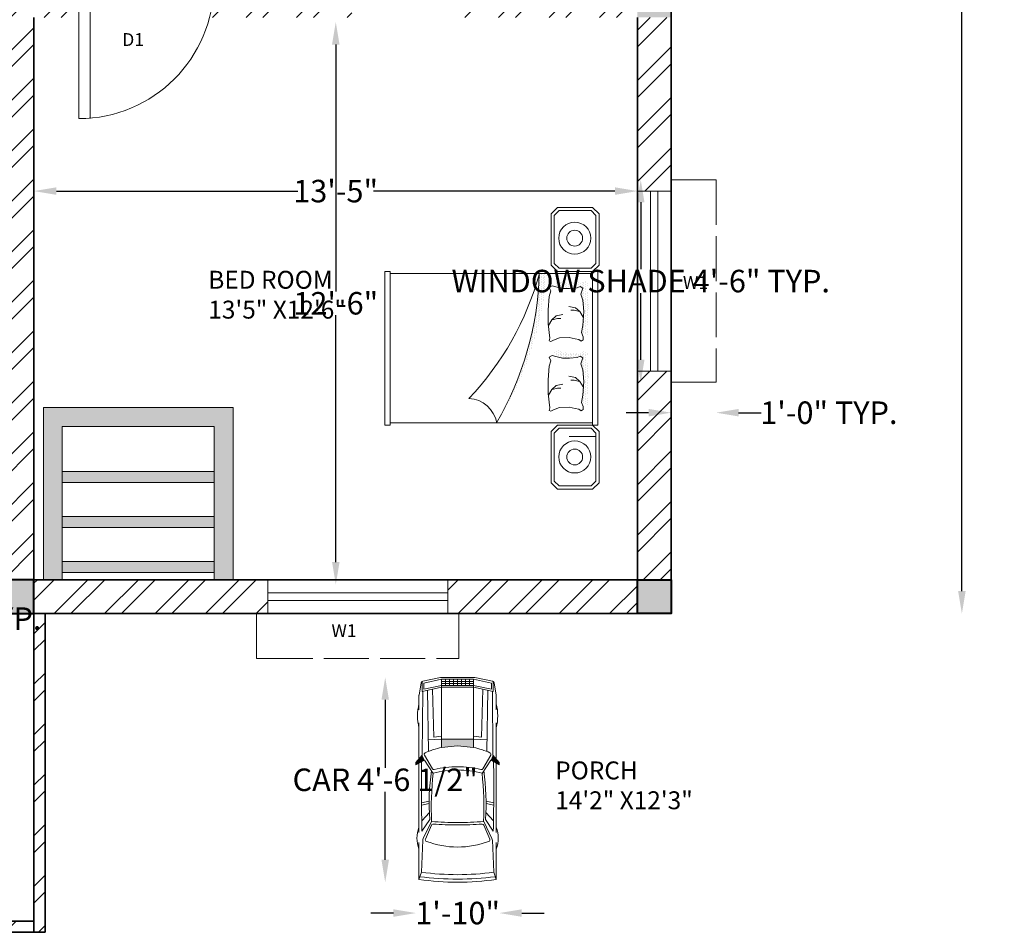
# Model space of a CAD drawing. Units: inches. Extents: x 3614 to 4242, y 2406 to 3033.
# Tile 9 of 10: x 3980 to 4242, y 2489 to 2733. Entities that reach past the tile are written whole.
import ezdxf

# ---------------------------------------------------------------- set-up
doc = ezdxf.new("R2010")
doc.units = ezdxf.units.IN
doc.linetypes.add('ACAD_ISO02W100', pattern=[15, 12, -3])
for name, color, linetype, lineweight in [('A-ANNO-DIMS', 2, 'Continuous', 18), ('A-ANNO-TEXT', 7, 'Continuous', 18), ('A-AREA-IDEN', 7, 'Continuous', 25), ('A-COLS', 7, 'Continuous', 40), ('A-COLS-PATT', 252, 'Continuous', 18), ('A-DOOR', 3, 'Continuous', 18), ('A-EQPM', 8, 'Continuous', 18), ('A-FURN', 8, 'Continuous', 18), ('A-FURN-PATT', 252, 'Continuous', 13), ('A-GLAZ', 4, 'Continuous', 18), ('A-GLAZ-OVHD', 8, 'ACAD_ISO02W100', 13), ('A-WALL', 7, 'Continuous', 35), ('A-WALL-PATT', 252, 'Continuous', 13)]:
    doc.layers.add(name, color=color, linetype=linetype, lineweight=lineweight)
doc.styles.add('ATTR', font='romans.shx', dxfattribs={"width": 0.8, "height": 1.114828})
doc.styles.get("Standard").update_dxf_attribs({"font": 'arial.ttf'})
doc.dimstyles.get("Standard").update_dxf_attribs({"dimtxt": 6, "dimasz": 6, "dimexe": 0.18, "dimexo": 0.0625, "dimgap": 0.09, "dimtad": 0, "dimtih": 1, "dimtoh": 1, "dimdec": 4, "dimzin": 0, "dimdsep": 46, "dimlunit": 4, "dimtxsty": 'Standard', "dimcen": 0.09, "dimse1": 1, "dimse2": 1, "dimadec": 0, "dimazin": 0, "dimtfac": 1, "dimtdec": 4, "dimtofl": 0, "dimtmove": 0, "dimatfit": 3, "dimfxl": 1, "dimtolj": 1, "dimtzin": 0, "dimarcsym": 0})
pattern_1 = [(270, (-3578.6833, 5895.14276), (0.451673685, -0.225836843), [0, -0.451673685])]

# ---------------------------------------------------------------- blocks, each defined once
blk = doc.blocks.new('*D19')
at = {"layer": 'A-ANNO-DIMS', "color": 0, "lineweight": -2, "transparency": 16777216}
for p, q in [((4063.88, 2726.09), (4063.88, 2660.24)), ((4063.88, 2588.09), (4063.88, 2653.94))]:
    blk.add_line(p, q, dxfattribs=at)
at = {"layer": 'A-ANNO-DIMS', "color": 0, "transparency": 16777216}
for points in [[(4062.88, 2726.09), (4064.88, 2726.09), (4063.88, 2732.09)], [(4062.88, 2588.09), (4064.88, 2588.09), (4063.88, 2582.09)]]:
    blk.add_solid(points, dxfattribs=at)
at = {"layer": 'Defpoints', "color": 0, "transparency": 16777216}
for p in [(4096.83, 2732.09), (4063.88, 2582.09), (4096.83, 2582.09)]:
    blk.add_point(p, dxfattribs=at)
at = {"layer": 'A-ANNO-DIMS', "color": 0, "transparency": 16777216, "insert": (4063.88, 2657.09), "char_height": 6, "attachment_point": 5}
blk.add_mtext('\\A1;12\'-6"', dxfattribs=at)
blk = doc.blocks.new('*D20')
at = {"layer": 'A-ANNO-DIMS', "color": 0, "lineweight": -2, "transparency": 16777216}
for p, q in [((3989.34, 2687.01), (4053.72, 2687.01)), ((4138.34, 2687.01), (4073.95, 2687.01))]:
    blk.add_line(p, q, dxfattribs=at)
at = {"layer": 'A-ANNO-DIMS', "color": 0, "transparency": 16777216}
for points in [[(3989.34, 2688.01), (3989.34, 2686.01), (3983.34, 2687.01)], [(4138.34, 2688.01), (4138.34, 2686.01), (4144.34, 2687.01)]]:
    blk.add_solid(points, dxfattribs=at)
at = {"layer": 'Defpoints', "color": 0, "transparency": 16777216}
for p in [(3983.34, 2692), (4144.34, 2692), (4144.34, 2687.01)]:
    blk.add_point(p, dxfattribs=at)
at = {"layer": 'A-ANNO-DIMS', "color": 0, "transparency": 16777216, "insert": (4063.84, 2687.01), "char_height": 6, "attachment_point": 5}
blk.add_mtext('\\A1;13\'-5"', dxfattribs=at)
blk = doc.blocks.new('A$C682073C8')
for p, q in [((-1.51, 0.58), (-1.388, 0.684)), ((-1.428, 0.543), (-1.348, 0.684)), ((-1.388, 0.684), (-1.348, 0.684)), ((-2.78, 0.282), (-2.724, 0.571)), ((-2.69, 0.555), (-2.752, 0.263)), ((-2.554, 0.581), (-2.72, 0.581)), ((-2.694, 0.6), (-2.493, 0.633)), ((-2.59, 0.555), (-2.69, 0.555)), ((-2.59, 0.555), (-2.652, 0.263)), ((-2.554, 0.581), (-2.622, 0.263)), ((-1.57, 0.478), (-2.572, 0.496)), ((-2.557, 0.57), (-1.51, 0.58)), ((-2.251, 0.635), (-2.478, 0.635)), ((-1.445, 0.635), (-2.04, 0.635)), ((-1.286, 0.414), (-1.508, 0.544)), ((-1.209, 0.401), (-1.428, 0.543)), ((-0.237, 0.635), (-1.376, 0.635)), ((-0.755, 0.467), (-0.727, 0.593)), ((-0.714, 0.467), (-0.686, 0.593)), ((-0.432, 0.589), (-0.565, 0.464)), ((-0.451, 0.457), (-0.263, 0.585)), ((-0.142, 0.564), (-0.42, 0.428)), ((-0.361, 0.431), (-0.128, 0.528)), ((0.411, 0.593), (-0.11, 0.572)), ((0.532, 0.635), (-0.072, 0.635)), ((0.532, 0.635), (0.411, 0.593)), ((-1.805, 0.393), (-2.59, 0.413)), ((-1.818, 0.263), (-1.805, 0.393)), ((-1.771, 0.263), (-1.758, 0.481)), ((-2.781, 0), (-2.781, 0.273)), ((-2.752, 0.263), (-2.752, 0)), ((-1.633, 0.263), (-2.752, 0.263)), ((-2.652, 0.197), (-2.752, 0.197)), ((-2.718, 0.263), (-2.718, 0)), ((-2.685, 0.263), (-2.685, 0)), ((-2.652, 0.263), (-2.652, 0)), ((-2.622, 0.263), (-2.622, 0)), ((-1.771, 0.263), (-1.771, 0)), ((-1.633, 0.263), (-1.659, 0)), ((-2.781, 0), (-2.781, -0.273)), ((-2.652, 0.132), (-2.752, 0.132)), ((-2.652, 0.066), (-2.752, 0.066)), ((-2.652, 0), (-2.752, 0)), ((-2.752, -0.263), (-2.752, 0)), ((-2.718, -0.263), (-2.718, 0)), ((-2.685, -0.263), (-2.685, 0)), ((-2.652, -0.263), (-2.652, 0)), ((-2.622, -0.263), (-2.622, 0)), ((-1.771, -0.263), (-1.771, 0)), ((-1.659, 0), (-1.633, -0.263)), ((-2.652, -0.066), (-2.752, -0.066)), ((-2.652, -0.132), (-2.752, -0.132)), ((-2.78, -0.282), (-2.724, -0.571)), ((-2.652, -0.197), (-2.752, -0.197)), ((-1.633, -0.263), (-2.752, -0.263)), ((-2.69, -0.555), (-2.752, -0.263)), ((-2.59, -0.555), (-2.652, -0.263)), ((-2.554, -0.581), (-2.622, -0.263)), ((-1.818, -0.263), (-1.805, -0.393)), ((-1.771, -0.263), (-1.758, -0.481)), ((-1.805, -0.393), (-2.59, -0.413)), ((-1.57, -0.478), (-2.572, -0.496)), ((-1.286, -0.414), (-1.508, -0.544)), ((-1.209, -0.401), (-1.428, -0.543)), ((-0.755, -0.467), (-0.727, -0.593)), ((-0.714, -0.467), (-0.686, -0.593)), ((-0.432, -0.589), (-0.565, -0.464)), ((-0.451, -0.457), (-0.263, -0.585)), ((-0.142, -0.564), (-0.42, -0.428)), ((-0.361, -0.431), (-0.128, -0.528)), ((-2.554, -0.581), (-2.72, -0.581)), ((-2.694, -0.6), (-2.493, -0.633)), ((-2.59, -0.555), (-2.69, -0.555)), ((-2.557, -0.57), (-1.51, -0.58)), ((-2.251, -0.635), (-2.478, -0.635)), ((-1.445, -0.635), (-2.04, -0.635)), ((-1.51, -0.58), (-1.388, -0.684)), ((-1.428, -0.543), (-1.348, -0.684)), ((-0.237, -0.635), (-1.376, -0.635)), ((0.411, -0.593), (-0.11, -0.572)), ((0.532, -0.635), (-0.072, -0.635)), ((0.532, -0.635), (0.411, -0.593)), ((-1.388, -0.684), (-1.348, -0.684))]:
    blk.add_line(p, q)
for centre, radius, start, end in [((-2.154, -0.189), 0.847, 76.4679, 103.5321), ((-0.146, 0.162), 0.505, 69.2613, 110.7387), ((-2.688, 0.564), 0.0366, 99.5555, 168.9219), ((-2.478, 0.542), 0.0932, 90, 99.5555), ((-0.341, 0), 1.319, 156.2323, 168.4871), ((-1.522, 0.52), 0.0277, 59.6014, 156.2323), ((-0.97, -26.413), 27.007, 88.4985, 90.9138), ((-0.106, 0.49), 0.0817, 92.3222, 116.0777), ((-0.118, 0.504), 0.0264, 20.6689, 112.6283), ((-1.453, 0), 1.453, 360, 20.6689), ((-3.642, 0), 4.096, 360, 8.3245), ((-4.512, 0), 5.038, 360, 7.0662), ((-3.75, 0), 4.328, 360, 8.4328), ((0.324, 0), 1.642, 166.5017, 180), ((-1.3, 0.39), 0.0277, 346.5017, 59.6014), ((0.222, 0), 1.487, 164.3473, 180), ((-0.728, -3.189), 3.656, 85.6618, 98.2609), ((-0.642, -4.704), 5.136, 87.5218, 96.3432), ((-5.551, 0), 5.149, 360, 4.7655), ((-0.35, 0.407), 0.0264, 112.6283, 183.982), ((-6.195, 0), 5.833, 360, 3.982), ((-2.736, 0.273), 0.045, 168.9219, 180), ((0.324, 0), 1.642, 180, 193.4983), ((0.222, 0), 1.487, 180, 195.6527), ((-5.551, 0), 5.149, 355.2345, 360), ((-6.195, 0), 5.833, 356.018, 360), ((-1.453, 0), 1.453, 339.3311, 360), ((-3.642, 0), 4.096, 351.6755, 360), ((-4.512, 0), 5.038, 352.9338, 360), ((-3.75, 0), 4.328, 351.5672, 360), ((-2.736, -0.273), 0.045, 180, 191.0781), ((-0.341, 0), 1.319, 191.5129, 203.7677), ((-1.3, -0.39), 0.0277, 300.3986, 13.4983), ((-0.728, 3.189), 3.656, 261.7391, 274.3382), ((-0.642, 4.704), 5.136, 263.6568, 272.4781), ((-0.35, -0.407), 0.0264, 176.018, 247.3717), ((-2.688, -0.564), 0.0366, 191.0781, 260.4445), ((-2.478, -0.542), 0.0932, 260.4445, 270), ((-2.154, 0.189), 0.847, 256.4679, 283.5321), ((-1.522, -0.52), 0.0277, 203.7677, 300.3986), ((-0.97, 26.413), 27.007, 269.0862, 271.5015), ((-0.146, -0.162), 0.505, 249.2613, 290.7387), ((-0.106, -0.49), 0.0817, 243.9223, 267.6778), ((-0.118, -0.504), 0.0264, 247.3717, 339.3311)]:
    blk.add_arc(centre, radius, start, end)
for points in [[(-1.428, 0.543), (-1.51, 0.58), (-1.348, 0.684), (-1.388, 0.684)], [(-1.633, 0.263), (-1.659, 0), (-1.771, 0.263), (-1.771, -0.263)], [(-1.659, 0), (-1.633, -0.263), (-1.771, -0.263)], [(-1.428, -0.543), (-1.51, -0.58), (-1.348, -0.684), (-1.388, -0.684)]]:
    blk.add_solid(points)
at = {"style": 'ATTR', "width": 0.8, "flags": 9}
blk.add_attdef('ESTCODE', (-2.781, 0), '', height=0.00071, rotation=180, dxfattribs=at)
blk = doc.blocks.new('*D25')
at = {"layer": 'A-ANNO-DIMS', "color": 0, "lineweight": -2, "transparency": 16777216}
for p, q in [((4230.92, 2948.34), (4230.92, 2767.5)), ((4230.92, 2580.34), (4230.92, 2761.19))]:
    blk.add_line(p, q, dxfattribs=at)
at = {"layer": 'A-ANNO-DIMS', "color": 0, "transparency": 16777216}
for points in [[(4229.92, 2948.34), (4231.92, 2948.34), (4230.92, 2954.34)], [(4229.92, 2580.34), (4231.92, 2580.34), (4230.92, 2574.34)]]:
    blk.add_solid(points, dxfattribs=at)
at = {"layer": 'Defpoints', "color": 0, "transparency": 16777216}
for p in [(4153.34, 2954.34), (4153.34, 2574.34), (4230.92, 2574.34)]:
    blk.add_point(p, dxfattribs=at)
at = {"layer": 'A-ANNO-DIMS', "color": 0, "transparency": 16777216, "insert": (4230.92, 2764.34), "char_height": 6, "attachment_point": 5}
blk.add_mtext('\\A1;31\'-8"', dxfattribs=at)
blk = doc.blocks.new('WINDOW-W1-48IN')
for p, q in [((48, 9), (0, 9)), ((0, 9), (0, 0)), ((48, 0), (48, 9)), ((0, 5.5), (48, 5.5)), ((0, 3.5), (48, 3.5)), ((0, 0), (48, 0))]:
    blk.add_line(p, q)
blk = doc.blocks.new('SHADE-W1')
for p, q in [((0, 0), (0, 12)), ((0, 12), (51, 12)), ((51, 12), (54, 12)), ((54, 12), (54, 0)), ((3, 0), (0, 0))]:
    blk.add_line(p, q)
blk = doc.blocks.new('COLUMN-9X9')
blk.add_lwpolyline([(9, 9), (0, 9), (0, 0), (9, 0)], close=True)
blk = doc.blocks.new('DOOR-SWING-36IN')
for p, q in [((0, 36), (0, 0)), ((0, 0), (0, 36)), ((3, 0), (3, 36))]:
    blk.add_line(p, q)
blk.add_arc((0, 36), 36, 270, 0)
blk = doc.blocks.new('BED-DOUBLE-WITH-NIGHTSTANDS')
h = blk.add_hatch()
h.set_pattern_fill('DOTS', color=256, scale=0.284519, angle=-90, style=0)
h.set_pattern_definition(pattern_1)
h.paths.add_polyline_path([(43.21, 57.47), (41.26, 57.47, -0.124273), (29.87, 17.64, 0.122563)])
h = blk.add_hatch()
h.set_pattern_fill('DOTS', color=256, scale=0.284519, angle=-90, style=0)
h.set_pattern_definition(pattern_1)
h.paths.add_polyline_path([(53.82, 40.86), (54.34, 41.21), (54.34, 42), (53.9, 43.14), (54.25, 45.06), (54.52, 48.74), (54.25, 51.8), (53.73, 53.38), (54.25, 55.04), (53.55, 55.48), (52.77, 55.13), (50.75, 54.95), (48.83, 54.95), (47.08, 55.39), (46.12, 55.65), (45.33, 55.22), (45.77, 54.25), (45.69, 53.96), (47.41, 53.53), (49.34, 53.53), (51.35, 53.71), (52.13, 54.06), (52.83, 53.62), (52.31, 51.96), (52.83, 50.38), (53.1, 47.32), (52.83, 43.64), (52.48, 41.72), (52.6, 41.41), (53.2, 41.3)])
h.paths.add_polyline_path([(53.82, 22.27), (54.34, 22.62), (54.34, 23.41), (53.9, 24.55), (54.25, 26.48), (54.52, 30.15), (54.25, 33.21), (53.73, 34.79), (54.25, 36.45), (53.55, 36.89), (52.77, 36.54), (50.75, 36.37), (48.83, 36.37), (47.08, 36.8), (46.12, 37.07), (45.33, 36.63), (45.77, 35.67), (45.69, 35.38), (47.41, 34.95), (49.34, 34.95), (51.35, 35.12), (52.13, 35.47), (52.83, 35.03), (52.31, 33.37), (52.83, 31.79), (53.1, 28.73), (52.83, 25.05), (52.48, 23.13), (52.6, 22.82), (53.2, 22.71)])
for p, q in [((0, 17.07), (0, 58.04)), ((0, 58.04), (1.42, 58.04)), ((1.42, 17.07), (1.42, 58.04)), ((55.48, 17.07), (55.48, 58.04)), ((55.48, 58.04), (56.9, 58.04)), ((56.9, 17.07), (56.9, 58.04)), ((1.42, 57.47), (55.48, 57.47)), ((1.42, 17.07), (0, 17.07)), ((55.48, 17.64), (1.42, 17.64)), ((56.9, 17.07), (55.48, 17.07)), ((56.3, 14.01), (49.19, 14.01))]:
    blk.add_line(p, q)
for points in [[(44.39, 73.41), (44.39, 59.75), (46.09, 58.04), (55.48, 58.04), (57.19, 59.75), (57.19, 73.41), (55.48, 75.11), (46.09, 75.11)], [(45.24, 72.98), (45.24, 60.18), (46.52, 58.9), (55.05, 58.9), (56.33, 60.18), (56.33, 72.98), (55.05, 74.26), (46.52, 74.26)], [(44.39, 15.36), (44.39, 1.71), (46.09, 0), (55.48, 0), (57.19, 1.71), (57.19, 15.36), (55.48, 17.07), (46.09, 17.07)], [(45.24, 14.94), (45.24, 2.13), (46.52, 0.85), (55.05, 0.85), (56.33, 2.13), (56.33, 14.94), (55.05, 16.22), (46.52, 16.22)]]:
    blk.add_lwpolyline(points, close=True)
for points in [[(52.31, 51.96), (52.83, 53.62), (52.13, 54.06), (51.35, 53.71), (49.34, 53.53), (47.41, 53.53), (45.66, 53.97), (44.7, 54.23), (43.91, 53.8), (44.35, 52.83), (43.91, 51.34), (43.65, 47.76), (43.65, 44.08), (44.09, 40.23), (43.91, 39.53), (44.35, 39.35), (45.05, 39.7), (46.62, 40.32), (49.25, 40.4), (50.82, 40.05), (51.78, 39.88), (52.4, 39.44), (52.92, 39.79), (52.92, 40.58), (52.48, 41.72), (52.83, 43.64), (53.1, 47.32), (52.83, 50.38), (52.31, 51.96)], [(52.92, 45.83), (52.05, 47.32), (50.91, 48.37), (49.16, 48.72)], [(51.96, 47.32), (50.56, 47.67), (49.69, 47.67)], [(43.74, 43.64), (44.61, 45.13), (45.75, 46.18), (47.5, 46.53)], [(44.7, 45.13), (46.1, 45.48), (46.97, 45.48)], [(52.31, 33.37), (52.83, 35.03), (52.13, 35.47), (51.35, 35.12), (49.34, 34.95), (47.41, 34.95), (45.66, 35.38), (44.7, 35.65), (43.91, 35.21), (44.35, 34.24), (43.91, 32.76), (43.65, 29.17), (43.65, 25.49), (44.09, 21.64), (43.91, 20.94), (44.35, 20.77), (45.05, 21.12), (46.62, 21.73), (49.25, 21.82), (50.82, 21.47), (51.78, 21.29), (52.4, 20.85), (52.92, 21.2), (52.92, 21.99), (52.48, 23.13), (52.83, 25.05), (53.1, 28.73), (52.83, 31.79), (52.31, 33.37)], [(52.92, 27.24), (52.05, 28.73), (50.91, 29.78), (49.16, 30.13)], [(51.96, 28.73), (50.56, 29.08), (49.69, 29.08)], [(43.74, 25.05), (44.61, 26.54), (45.75, 27.59), (47.5, 27.94)], [(44.7, 26.54), (46.1, 26.89), (46.97, 26.89)]]:
    blk.add_lwpolyline(points)
for centre, radius in [((50.7, 66.92), 4.27), ((50.7, 66.92), 2.11), ((50.7, 8.56), 4.27), ((50.7, 8.56), 2.11)]:
    blk.add_circle(centre, radius)
for centre, radius, start, end in [((-34.21, 78.09), 78.23, 316.4367, 344.7234), ((-43.33, 60.1), 84.62, 329.8866, 358.2226), ((22.03, 16.21), 7.98, 10.3543, 86.7862)]:
    blk.add_arc(centre, radius, start, end)
blk = doc.blocks.new('*D39')
at = {"layer": 'A-ANNO-DIMS', "color": 0, "lineweight": -2, "transparency": 16777216}
for p, q in [((3884.34, 2572.99), (3878.34, 2572.99)), ((3905.34, 2572.99), (3911.34, 2572.99))]:
    blk.add_line(p, q, dxfattribs=at)
at = {"layer": 'A-ANNO-DIMS', "color": 0, "transparency": 16777216}
for points in [[(3884.34, 2573.99), (3884.34, 2571.99), (3890.34, 2572.99)], [(3905.34, 2573.99), (3905.34, 2571.99), (3899.34, 2572.99)]]:
    blk.add_solid(points, dxfattribs=at)
at = {"layer": 'Defpoints', "color": 0, "transparency": 16777216}
for p in [(3890.34, 2574.34), (3899.34, 2574.34), (3899.34, 2572.99)]:
    blk.add_point(p, dxfattribs=at)
at = {"layer": 'A-ANNO-DIMS', "color": 0, "transparency": 16777216, "insert": (3949, 2572.99), "char_height": 6, "attachment_point": 5}
blk.add_mtext('\\A1;COLUMN 0\'-9" TYP.', dxfattribs=at)
blk = doc.blocks.new('*D43')
at = {"layer": 'A-ANNO-DIMS', "color": 0, "lineweight": -2, "transparency": 16777216}
for p, q in [((4145.24, 2684.01), (4145.24, 2666.2)), ((4145.24, 2642.01), (4145.24, 2659.81))]:
    blk.add_line(p, q, dxfattribs=at)
at = {"layer": 'A-ANNO-DIMS', "color": 0, "transparency": 16777216}
for points in [[(4144.24, 2684.01), (4146.24, 2684.01), (4145.24, 2690.01)], [(4144.24, 2642.01), (4146.24, 2642.01), (4145.24, 2636.01)]]:
    blk.add_solid(points, dxfattribs=at)
at = {"layer": 'Defpoints', "color": 0, "transparency": 16777216}
for p in [(4153.34, 2690.01), (4145.24, 2636.01), (4153.34, 2636.01)]:
    blk.add_point(p, dxfattribs=at)
at = {"layer": 'A-ANNO-DIMS', "color": 0, "transparency": 16777216, "insert": (4145.24, 2663.01), "char_height": 6, "attachment_point": 5}
blk.add_mtext('\\A1;WINDOW SHADE 4\'-6" TYP.', dxfattribs=at)
blk = doc.blocks.new('*D44')
at = {"layer": 'A-ANNO-DIMS', "color": 0, "lineweight": -2, "transparency": 16777216}
for p, q in [((4147.34, 2627.91), (4141.34, 2627.91)), ((4171.34, 2627.91), (4177.34, 2627.91))]:
    blk.add_line(p, q, dxfattribs=at)
at = {"layer": 'A-ANNO-DIMS', "color": 0, "transparency": 16777216}
for points in [[(4147.34, 2628.91), (4147.34, 2626.91), (4153.34, 2627.91)], [(4171.34, 2628.91), (4171.34, 2626.91), (4165.34, 2627.91)]]:
    blk.add_solid(points, dxfattribs=at)
at = {"layer": 'Defpoints', "color": 0, "transparency": 16777216}
for p in [(4153.34, 2636.01), (4165.34, 2636.01), (4165.34, 2627.91)]:
    blk.add_point(p, dxfattribs=at)
at = {"layer": 'A-ANNO-DIMS', "color": 0, "transparency": 16777216, "insert": (4195.43, 2627.91), "char_height": 6, "attachment_point": 5}
blk.add_mtext('\\A1;1\'-0" TYP.', dxfattribs=at)
blk = doc.blocks.new('*D65')
at = {"layer": 'A-ANNO-DIMS', "color": 0, "lineweight": -2, "transparency": 16777216}
for p, q in [((4077.07, 2551.34), (4077.07, 2533.2)), ((4077.07, 2508.67), (4077.07, 2526.81))]:
    blk.add_line(p, q, dxfattribs=at)
at = {"layer": 'A-ANNO-DIMS', "color": 0, "transparency": 16777216}
for points in [[(4076.07, 2551.34), (4078.07, 2551.34), (4077.07, 2557.34)], [(4076.07, 2508.67), (4078.07, 2508.67), (4077.07, 2502.67)]]:
    blk.add_solid(points, dxfattribs=at)
at = {"layer": 'Defpoints', "color": 0, "transparency": 16777216}
for p in [(4085.27, 2557.34), (4077.07, 2502.67), (4085.27, 2502.67)]:
    blk.add_point(p, dxfattribs=at)
at = {"layer": 'A-ANNO-DIMS', "color": 0, "transparency": 16777216, "insert": (4077.07, 2530.01), "char_height": 6, "attachment_point": 5}
blk.add_mtext('\\A1;CAR 4\'-6 1/2"', dxfattribs=at)
blk = doc.blocks.new('*D66')
at = {"layer": 'A-ANNO-DIMS', "color": 0, "lineweight": -2, "transparency": 16777216}
for p, q in [((4079.27, 2494.47), (4073.27, 2494.47)), ((4113.49, 2494.47), (4119.49, 2494.47))]:
    blk.add_line(p, q, dxfattribs=at)
at = {"layer": 'A-ANNO-DIMS', "color": 0, "transparency": 16777216}
for points in [[(4079.27, 2495.47), (4079.27, 2493.47), (4085.27, 2494.47)], [(4113.49, 2495.47), (4113.49, 2493.47), (4107.49, 2494.47)]]:
    blk.add_solid(points, dxfattribs=at)
at = {"layer": 'Defpoints', "color": 0, "transparency": 16777216}
for p in [(4085.27, 2502.67), (4107.49, 2502.67), (4107.49, 2494.47)]:
    blk.add_point(p, dxfattribs=at)
at = {"layer": 'A-ANNO-DIMS', "color": 0, "transparency": 16777216, "insert": (4096.38, 2494.47), "char_height": 6, "attachment_point": 5}
blk.add_mtext('\\A1;1\'-10"', dxfattribs=at)

msp = doc.modelspace()

# ---------------------------------------------------------------- hatches: boundary and pattern name
at = {"layer": 'A-COLS-PATT'}
h = msp.add_hatch(color=256, dxfattribs=at)
h.dxf.hatch_style = 1
h.paths.add_polyline_path([(3697.336, 2954.34049), (3688.336, 2954.34049), (3688.336, 2945.34049), (3697.336, 2945.34049)])
h.paths.add_polyline_path([(3818.336, 2954.34049), (3809.336, 2954.34049), (3809.336, 2945.34049), (3818.336, 2945.34049)])
h.paths.add_polyline_path([(3818.336, 2787.28572), (3809.336, 2787.28572), (3809.336, 2778.34049), (3818.336, 2778.34049)])
h.paths.add_polyline_path([(3697.336, 2742.34049), (3688.336, 2742.34049), (3688.336, 2733.34049), (3697.336, 2733.34049)])
h.paths.add_polyline_path([(3697.336, 2583.37355), (3688.336, 2583.37355), (3688.336, 2574.37355), (3697.336, 2574.37355)])
h.paths.add_polyline_path([(3899.336, 2583.34049), (3890.336, 2583.34049), (3890.336, 2574.34049), (3899.336, 2574.34049)])
h.paths.add_polyline_path([(3983.336, 2583.34049), (3974.336, 2583.34049), (3974.336, 2574.34049), (3983.336, 2574.34049)])
h.paths.add_polyline_path([(4153.336, 2583.34049), (4144.336, 2583.34049), (4144.336, 2574.34049), (4153.336, 2574.34049)])
h.paths.add_polyline_path([(4153.336, 2742.34049), (4144.336, 2742.34049), (4144.336, 2733.34049), (4153.336, 2733.34049)])
h.paths.add_polyline_path([(4153.336, 2795.34049), (4144.336, 2795.34049), (4144.336, 2786.34049), (4153.336, 2786.34049)])
h.paths.add_polyline_path([(3983.336, 2795.31105), (3974.336, 2795.31105), (3974.336, 2786.34049), (3983.336, 2786.34049)])
h.paths.add_polyline_path([(4153.336, 2954.34049), (4144.36882, 2954.34049), (4144.36882, 2945.34049), (4153.336, 2945.34049)])
h.paths.add_polyline_path([(3982.96188, 2954.34049), (3973.96188, 2954.34049), (3973.96188, 2945.34049), (3982.96188, 2945.34049)])
at = {"layer": 'A-FURN-PATT'}
h = msp.add_hatch(color=256, dxfattribs=at)
h.dxf.hatch_style = 1
h.paths.add_polyline_path([(4036.46152, 2629.25932), (3998.22484, 2629.25932), (3985.86547, 2629.25932), (3985.86547, 2583.34049), (3990.86547, 2583.34049), (3990.86547, 2624.25932), (4031.46152, 2624.25932), (4031.46152, 2583.34049), (4036.46152, 2583.34049)])
h.paths.add_polyline_path([(4031.46152, 2612.25932), (3990.86547, 2612.25932), (3990.86547, 2609.25932), (4031.46152, 2609.25932)], flags=17)
h.paths.add_polyline_path([(4031.46152, 2600.25932), (3990.86547, 2600.25932), (3990.86547, 2597.25932), (4031.46152, 2597.25932)], flags=17)
h.paths.add_polyline_path([(4031.46152, 2588.25932), (3990.86547, 2588.25932), (3990.86547, 2585.25932), (4031.46152, 2585.25932)], flags=17)
at = {"layer": 'A-WALL-PATT'}
h = msp.add_hatch(dxfattribs=at)
h.set_pattern_fill('ANSI32', color=256)
h.paths.add_polyline_path([(3899.336, 2733.34049), (3899.336, 2742.34049), (3890.336, 2742.34049), (3890.336, 2583.34049), (3899.336, 2583.34049)])
h.paths.add_polyline_path([(3983.336, 2733.34049), (3995.336, 2733.34049), (3995.336, 2742.34049), (3983.336, 2742.34049), (3974.336, 2742.34049), (3974.336, 2583.34049), (3983.336, 2583.34049)])
h.paths.add_polyline_path([(3974.336, 2583.34049), (3899.336, 2583.34049), (3899.336, 2574.34049), (3974.336, 2574.34049)])
h.paths.add_polyline_path([(4045.73114, 2583.34049), (3983.336, 2583.34049), (3983.336, 2574.34049), (4045.73114, 2574.34049)])
h.paths.add_polyline_path([(4144.336, 2583.34049), (4093.73114, 2583.34049), (4093.73114, 2574.34049), (4144.336, 2574.34049)])
h.paths.add_polyline_path([(4153.336, 2639.00845), (4144.336, 2639.00845), (4144.336, 2583.34049), (4153.336, 2583.34049)])
h.paths.add_polyline_path([(4153.336, 2733.34049), (4144.336, 2733.34049), (4144.336, 2687.00845), (4153.336, 2687.00845)])
h.paths.add_polyline_path([(4144.336, 2742.34049), (4096.76112, 2742.34049, -0.076320834), (4098.14294, 2733.34049), (4144.336, 2733.34049)])
h.paths.add_polyline_path([(4068.14294, 2742.34049), (4056.14294, 2742.34049), (4031.336, 2742.34049, -0.063254224), (4030.19285, 2733.34049), (4068.14294, 2733.34049)])
h.paths.add_polyline_path([(4144.336, 2795.34049), (4042.336, 2795.34049), (4042.336, 2786.34049), (4144.336, 2786.34049)])
h.paths.add_polyline_path([(4153.336, 2854.95478), (4144.336, 2854.95478), (4144.336, 2795.34049), (4153.336, 2795.34049)])
h = msp.add_hatch(dxfattribs=at)
h.set_pattern_fill('ANSI32', color=256)
h.paths.add_polyline_path([(3983.336, 2492.34049), (3891.47836, 2492.34049), (3891.47836, 2489.34049), (3983.336, 2489.34049)])
h.paths.add_polyline_path([(3986.336, 2574.34049), (3983.336, 2574.34049), (3983.336, 2492.34049), (3983.336, 2489.34049), (3986.336, 2489.34049)])

# ---------------------------------------------------------------- linework, layer by layer
at = {"layer": 'A-FURN'}
for p, q in [((3985.86547, 2583.34049), (3985.86547, 2629.25932)), ((3985.86547, 2629.25932), (3998.22484, 2629.25932)), ((3998.22484, 2629.25932), (4036.46152, 2629.25932)), ((4036.46152, 2629.25932), (4036.46152, 2583.34049)), ((3990.86547, 2583.34049), (3990.86547, 2624.25932)), ((3990.86547, 2624.25932), (4031.46152, 2624.25932)), ((4031.46152, 2624.25932), (4031.46152, 2583.34049)), ((3990.86547, 2612.25932), (4031.46152, 2612.25932)), ((3990.86547, 2609.25932), (4031.46152, 2609.25932)), ((3990.86547, 2600.25932), (4031.46152, 2600.25932)), ((3990.86547, 2597.25932), (4031.46152, 2597.25932)), ((3990.86547, 2588.25932), (4031.46152, 2588.25932)), ((3990.86547, 2585.25932), (4031.46152, 2585.25932))]:
    msp.add_line(p, q, dxfattribs=at)
at = {"layer": 'A-GLAZ-OVHD'}
for p, q in [((4045.73114, 2574.34049), (4042.73114, 2574.34049)), ((4042.73114, 2574.34049), (4042.73114, 2562.34049)), ((4096.73114, 2562.34049), (4096.73114, 2574.34049)), ((4042.73114, 2562.34049), (4045.73114, 2562.34049)), ((4045.73114, 2562.34049), (4093.73114, 2562.34049)), ((4093.73114, 2562.34049), (4096.73114, 2562.34049))]:
    msp.add_line(p, q, dxfattribs=at)
at = {"layer": 'A-WALL'}
for p, q in [((4153.336, 2954.34049), (4153.336, 2574.34049)), ((3983.336, 2733.34049), (3983.336, 2583.34049)), ((4144.336, 2733.34049), (4144.336, 2583.34049)), ((4144.336, 2583.34049), (3983.336, 2583.34049)), ((4153.336, 2574.34049), (3974.336, 2574.34049)), ((3983.336, 2492.34049), (3983.336, 2574.34049)), ((3986.336, 2489.34049), (3986.336, 2574.34049)), ((3891.47836, 2492.34049), (3983.336, 2492.34049)), ((3983.336, 2492.34049), (3983.336, 2489.34049)), ((3891.47836, 2489.34049), (3986.336, 2489.34049))]:
    msp.add_line(p, q, dxfattribs=at)

# ---------------------------------------------------------------- block references
at = {"layer": 'A-COLS'}
msp.add_blockref('COLUMN-9X9', (3974.336, 2574.34), dxfattribs=at)
at = {"layer": 'A-COLS', "extrusion": (0, 0, -1), "zscale": -1, "rotation": 89.99999999999999}
msp.add_blockref('COLUMN-9X9', (-4144.33551, 2574.34049), dxfattribs=at)
at = {"layer": 'A-DOOR'}
msp.add_blockref('DOOR-SWING-36IN', (3995.336, 2706.34), dxfattribs=at)
at = {"layer": 'A-EQPM', "xscale": 16.25143296341211, "yscale": 16.25143296341211, "zscale": 16.25143296341211, "rotation": 270}
msp.add_blockref('A$C682073C8', (4096.38157, 2512.079), dxfattribs=at)
at = {"layer": 'A-FURN'}
msp.add_blockref('BED-DOUBLE-WITH-NIGHTSTANDS', (4076.93, 2607.539), dxfattribs=at)
at = {"layer": 'A-GLAZ', "extrusion": (0, 0, -1), "zscale": -1}
for p, rotation in [((-4144.33551, 2639.00875), 89.99999999999982), ((-4045.73144, 2583.34099), 180)]:
    msp.add_blockref('WINDOW-W1-48IN', p, dxfattribs=dict(at, rotation=rotation))
at = {"layer": 'A-GLAZ-OVHD', "rotation": 270.0000000000017}
msp.add_blockref('SHADE-W1', (4153.33551, 2690.00815), dxfattribs=at)

# ---------------------------------------------------------------- texts
at = {"layer": 'A-ANNO-TEXT', "char_height": 3.42604, "attachment_point": 1}
for s, insert in [('D1', (4006.90698, 2729.13284)), ('W1', (4156.49627, 2664.34453)), ('W1', (4062.72231, 2571.49311))]:
    msp.add_mtext_dynamic_manual_height_columns(s, width=192.8287007, gutter_width=17.1302, heights=[0], dxfattribs=dict(at, insert=insert))
at = {"layer": 'A-AREA-IDEN', "char_height": 4.7777047, "attachment_point": 1}
for s, width, gutter_width, insert in [('BED ROOM\\P13\'5" X12\'6"', 126.6171413, 23.88852, (4029.87162, 2665.74724)), ('PORCH\\P14\'2" X12\'3"', 66.2541682, 12.5, (4122.42043, 2534.90318))]:
    msp.add_mtext_dynamic_manual_height_columns(s, width=width, gutter_width=gutter_width, heights=[0], dxfattribs=dict(at, insert=insert))

# ---------------------------------------------------------------- dimensions: what is measured, and where the dimension line sits
at = {"layer": 'A-ANNO-DIMS'}
for base, p1, p2, picture, middle in [((4230.92276, 2574.34049), (4153.336, 2954.34049), (4153.336, 2574.34049), '*D25', (4230.92276, 2764.34049)), ((4063.87921, 2582.0893), (4096.82972, 2732.0893), (4096.82972, 2582.0893), '*D19', (4063.87921, 2657.0893))]:
    dim = msp.add_linear_dim(base=base, p1=p1, p2=p2, angle=90, dimstyle='Standard', override={"dimclrd": 0, "dimclre": 0, "dimclrt": 0}, dxfattribs=at)
    dim.commit()
    dim.dimension.update_dxf_attribs({"geometry": picture, "text_midpoint": middle})
for base, p1, p2, override, picture, middle in [((4144.336, 2687.00845), (3983.336, 2692.00064), (4144.336, 2692.00064), {"dimclrd": 0, "dimclre": 0, "dimclrt": 0}, '*D20', (4063.836, 2687.00845)), ((4107.49237, 2494.4736), (4085.27077, 2502.67341), (4107.49237, 2502.67341), {"dimdec": 1, "dimlfac": 1, "dimrnd": 0, "dimzin": 1, "dimdsep": 46, "dimlunit": 4, "dimfrac": 2}, '*D66', (4096.38157, 2494.4736))]:
    dim = msp.add_linear_dim(base=base, p1=p1, p2=p2, dimstyle='Standard', override=override, dxfattribs=at)
    dim.commit()
    dim.dimension.update_dxf_attribs({"geometry": picture, "text_midpoint": middle})
for base, p1, p2, angle, text, picture, middle in [((4145.236, 2636.00845), (4153.336, 2690.00845), (4153.336, 2636.00845), 270, 'WINDOW SHADE <> TYP.', '*D43', (4145.236, 2663.00845)), ((4165.336, 2627.90845), (4153.336, 2636.00845), (4165.336, 2636.00845), 0, '<> TYP.', '*D44', (4195.43009, 2627.90845)), ((4077.07097, 2502.67341), (4085.27077, 2557.33877), (4085.27077, 2502.67341), 270, 'CAR <>', '*D65', (4077.07097, 2530.00609))]:
    dim = msp.add_linear_dim(base=base, p1=p1, p2=p2, angle=angle, text=text, dimstyle='Standard', override={"dimdec": 1, "dimlfac": 1, "dimrnd": 0, "dimzin": 1, "dimdsep": 46, "dimlunit": 4, "dimfrac": 2}, dxfattribs=at)
    dim.commit()
    dim.dimension.update_dxf_attribs({"geometry": picture, "text_midpoint": middle})
dim = msp.add_linear_dim(base=(3899.336, 2572.99049), p1=(3890.336, 2574.34049), p2=(3899.336, 2574.34049), text='COLUMN <> TYP.', dimstyle='Standard', override={"dimdec": 1, "dimlfac": 1, "dimrnd": 0, "dimzin": 1, "dimdsep": 46, "dimlunit": 4, "dimfrac": 2}, dxfattribs=at)
dim.commit()
dim.dimension.update_dxf_attribs({"geometry": '*D39', "text_midpoint": (3949.00376, 2572.99049)})

doc.saveas('drawing.dxf')
